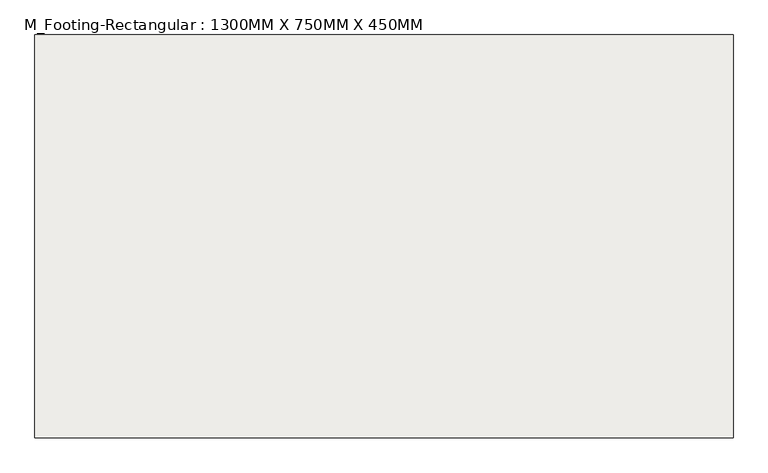
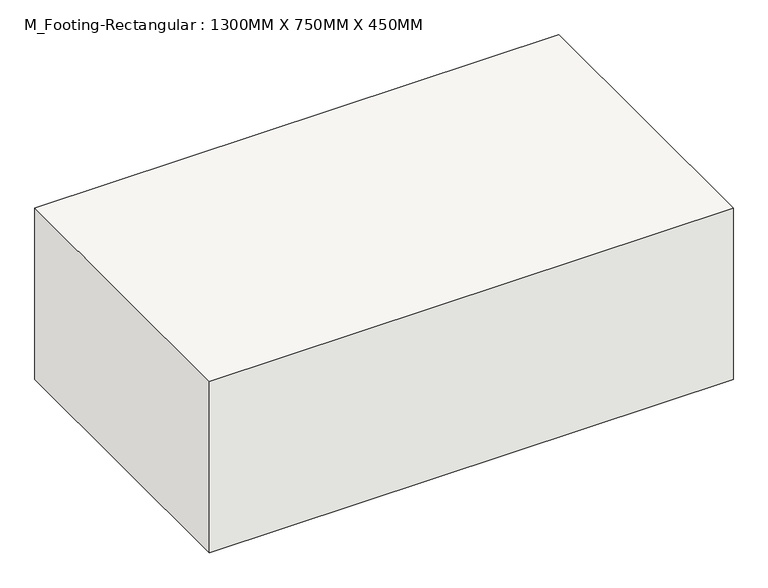
"""IFC4 building model written with IfcOpenShell, lengths in millimetres: slab geometry, M_Footing-Rectangular : 1300MM X 750MM X 450MM."""

from ifc_helpers import new_model, si_unit, frame, origin, place, context, project, spatial, polyline, outline, extrude, source, transform, mapped, element, save


def m_footing_rectangular_1300mm_x_750mm_x_450mm_70b2c142(model_context):
    return source(origin(), model_context, "Body", "SweptSolid", [
        extrude(outline(polyline([(650.0, 375.0), (650.0, -375.0), (-650.0, -375.0), (-650.0, 375.0), (650.0, 375.0)])), frame((0.0, 0.0, -450.0), z_axis=(0.0, 0.0, 1.0), x_axis=(1.0, 0.0, 0.0)), (0.0, 0.0, 1.0), 450.0),
    ])


if __name__ == "__main__":
    model = new_model("IFC4")
    model_context = context("Model", 3, world=origin())
    ifc_project = project(units=[si_unit("LENGTHUNIT", "METRE", prefix="MILLI")], contexts=[model_context])
    site = spatial("IfcSite", under=ifc_project)
    building = spatial("IfcBuilding", under=site)
    placement = place(None, origin())
    m_footing_rectangular_1300mm_x_750mm_x_450mm_shape = m_footing_rectangular_1300mm_x_750mm_x_450mm_70b2c142(model_context)
    element("IfcSlab", 1, ObjectType="M_Footing-Rectangular : 1300MM X 750MM X 450MM", at=placement, inside=building, context=model_context, shape_type="MappedRepresentation", body=[
        mapped(m_footing_rectangular_1300mm_x_750mm_x_450mm_shape, transform((0.0, 0.0, 0.0), x_axis=(1.0, 0.0, 0.0), y_axis=(0.0, 1.0, 0.0), z_axis=(0.0, 0.0, 1.0))),
    ])
    save(model, "model.ifc")

# Revit data of these elements
# Type "M_Footing-Rectangular : 1300MM X 750MM X 450MM"
#   Width = 1300 mm
#   Length = 750 mm
#   Foundation Thickness = 450 mm
#   Structural Material [instance default] = Concrete, Cast-in-Place gray
#   Assembly Code = ""
# Element 1 (IfcSlab, "M_Footing-Rectangular : 1300MM X 750MM X 450MM")
#   Materials on its faces: "Concrete, Cast-in-Place gray"
# Materials
#   "Concrete, Cast-in-Place gray": class "Concrete", colour RGB 192 192 192, transparency 0, Description = "Cast-in-place concrete", Cost = 0
